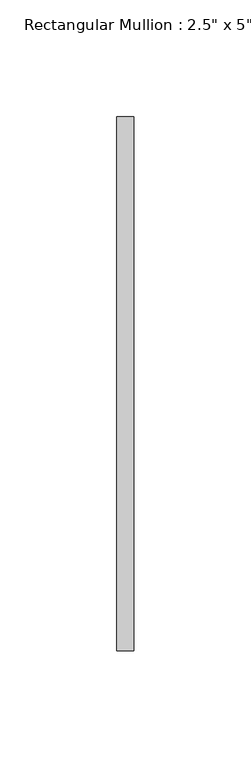
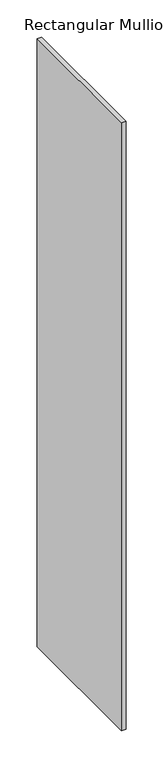
"""IFC4 building model written with IfcOpenShell, lengths in millimetres: member geometry."""

from ifc_helpers import new_model, si_unit, frame, origin, place, context, project, spatial, polyline, outline, extrude, source, transform, mapped, element, save


def member_cd12fca0(model_context):
    return source(origin(), model_context, "Body", "SweptSolid", [
        extrude(outline(polyline([(0.0, 114.3), (0.0, -114.3), (-7.239, -114.3), (-7.239, 114.3), (0.0, 114.3)])), frame((0.0, 0.0, -1003.3), z_axis=(0.0, 0.0, 1.0), x_axis=(1.0, 0.0, 0.0)), (0.0, 0.0, 1.0), 1003.3),
    ])


if __name__ == "__main__":
    model = new_model("IFC4")
    model_context = context("Model", 3, world=origin())
    ifc_project = project(units=[si_unit("LENGTHUNIT", "METRE", prefix="MILLI")], contexts=[model_context])
    site = spatial("IfcSite", under=ifc_project)
    building = spatial("IfcBuilding", under=site)
    placement = place(None, origin())
    member_shape = member_cd12fca0(model_context)
    element("IfcMember", 1, ObjectType="Rectangular Mullion : 2.5\" x 5\" rectangular", at=placement, inside=building, context=model_context, shape_type="MappedRepresentation", body=[
        mapped(member_shape, transform((0.0, 0.0, 0.0), x_axis=(1.0, 0.0, 0.0), y_axis=(0.0, 1.0, 0.0), z_axis=(0.0, 0.0, 1.0))),
    ])
    save(model, "model.ifc")

# Revit data of these elements
# Type "Rectangular Mullion : 2.5\" x 5\" rectangular"
#   built-in parameter 1007304 = 0.75 (stored number, unit not read)
#   built-in parameter 1007301 = 0.011875 (stored number, unit not read)
#   built-in parameter 1007300 = 0.011875 (stored number, unit not read)
# Element 1 (IfcMember, "Rectangular Mullion : 2.5\" x 5\" rectangular")
#   Materials on its faces: "WINDOW GLASS MATERIAL"
# Materials
#   "WINDOW GLASS MATERIAL": class "Generic", colour RGB 120 120 120, transparency 0, Cost = 0
